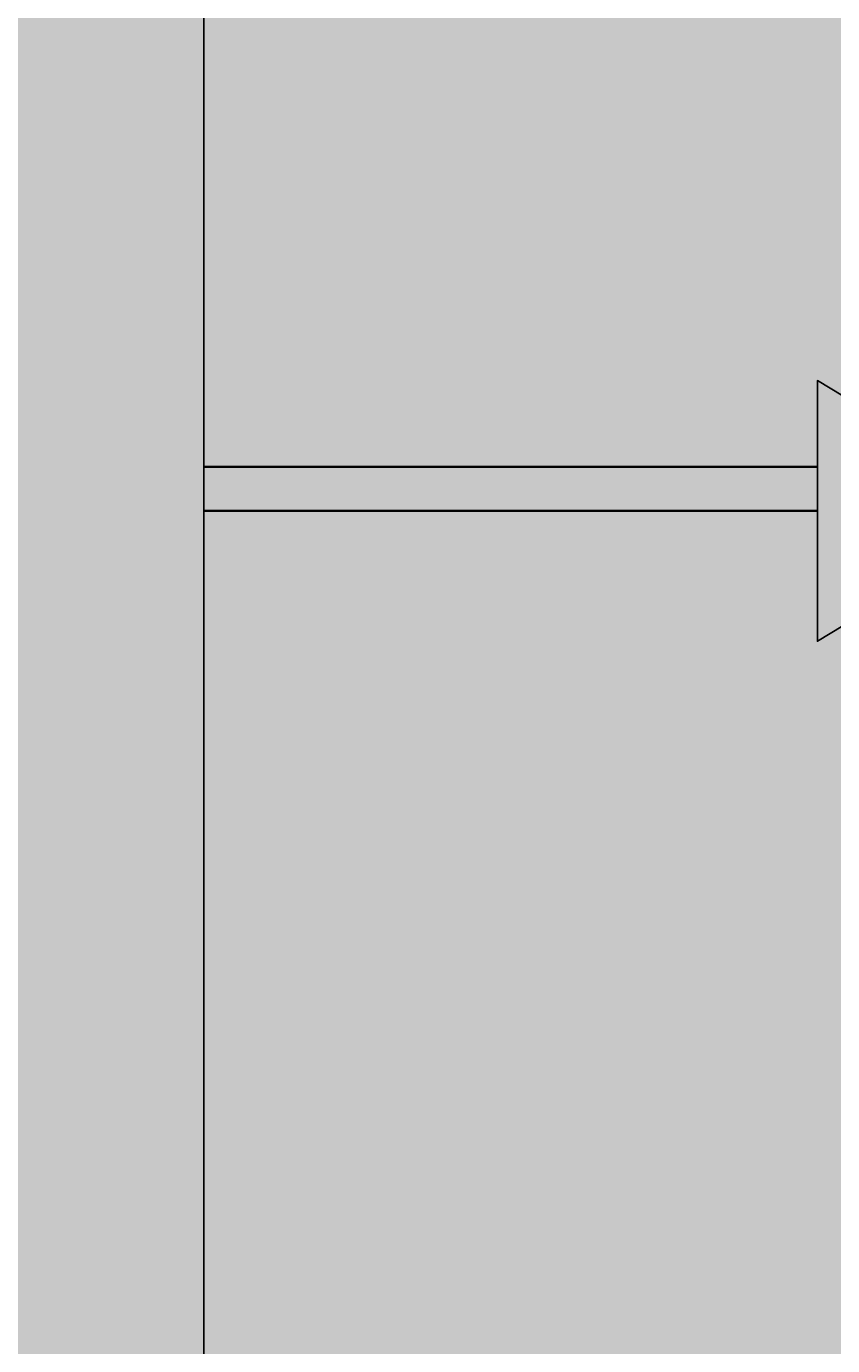
# Model space of a CAD drawing. Units: millimetres. Extents: x -22994 to 29398, y -19990 to 20176.
# Tile 57 of 135: x 198 to 216, y 65 to 95. Entities that reach past the tile are written whole.
import ezdxf
from ezdxf import colors
from ezdxf.entities.mleader import LeaderData, LeaderLine
from ezdxf.math import Vec2, Vec3

# ---------------------------------------------------------------- set-up
doc = ezdxf.new("R2010")
doc.units = ezdxf.units.MM
doc.header["$MEASUREMENT"] = 0
for name, color, linetype, lineweight in [('M-ANNO-TEXT', 7, 'Continuous', 25), ('M-DIMS', 2, 'Continuous', 18), ('M-EQPM', 7, 'Continuous', 25), ('M-EQPM-PATT', 7, 'Continuous', 18), ('M-PIPE', 7, 'Continuous', 35)]:
    doc.layers.add(name, color=color, linetype=linetype, lineweight=lineweight)
doc.styles.get("Standard").update_dxf_attribs({"font": 'arial.ttf'})
doc.dimstyles.get("Standard").update_dxf_attribs({"dimtxt": 0.18, "dimasz": 10000, "dimexe": 0.18, "dimexo": 0.0625, "dimgap": 0.09, "dimtad": 0, "dimtih": 1, "dimtoh": 1, "dimdec": 0, "dimzin": 0, "dimdsep": 46, "dimtxsty": 'Standard', "dimcen": 0.09, "dimadec": 0, "dimazin": 0, "dimtfac": 1, "dimtdec": 0, "dimtofl": 0, "dimtmove": 0, "dimatfit": 3, "dimfxl": 1, "dimtolj": 1, "dimtzin": 0, "dimlwd": 30, "dimarcsym": 0})

# ---------------------------------------------------------------- blocks, each defined once
blk = doc.blocks.new('*D2')
at = {"layer": 'Defpoints', "color": 0, "transparency": 16777216}
for p in [(6.677, 10.271), (290.852, 10.271), (290.852, -5.079)]:
    blk.add_point(p, dxfattribs=at)
at = {"layer": 'M-DIMS', "color": 0, "lineweight": -2, "transparency": 16777216}
for p, q in [((6.677, 10.209), (6.677, -5.259)), ((290.852, 10.209), (290.852, -5.259))]:
    blk.add_line(p, q, dxfattribs=at)
at = {"layer": 'M-DIMS', "color": 0, "lineweight": 30, "transparency": 16777216}
for p, q in [((-9993.323, -5.079), (-19993.323, -5.079)), ((10290.852, -5.079), (20290.852, -5.079))]:
    blk.add_line(p, q, dxfattribs=at)
at = {"layer": 'M-DIMS', "color": 0, "transparency": 16777216}
for points in [[(-9993.323, 1661.588), (-9993.323, -1671.745), (6.677, -5.079)], [(10290.852, 1661.588), (10290.852, -1671.745), (290.852, -5.079)]]:
    blk.add_solid(points, dxfattribs=at)
at = {"layer": 'M-DIMS', "color": 0, "transparency": 16777216, "insert": (148.765, -5.079), "char_height": 0.18, "attachment_point": 5}
blk.add_mtext('\\A1;284.2', dxfattribs=at)
blk = doc.blocks.new('*D3')
at = {"layer": 'Defpoints', "color": 0, "transparency": 16777216}
for p in [(110.265, 204.165), (110.265, 176.366), (95.833, 127.967)]:
    blk.add_point(p, dxfattribs=at)
at = {"layer": 'M-DIMS', "color": 0, "lineweight": -2, "transparency": 16777216}
for p, q in [((95.833, 128.03), (95.833, 204.345)), ((110.265, 176.429), (110.265, 204.345))]:
    blk.add_line(p, q, dxfattribs=at)
at = {"layer": 'M-DIMS', "color": 0, "lineweight": 30, "transparency": 16777216}
for p, q in [((-9904.167, 204.165), (-19904.167, 204.165)), ((10110.265, 204.165), (20110.265, 204.165))]:
    blk.add_line(p, q, dxfattribs=at)
at = {"layer": 'M-DIMS', "color": 0, "transparency": 16777216}
for points in [[(-9904.167, 1870.832), (-9904.167, -1462.501), (95.833, 204.165)], [(10110.265, 1870.832), (10110.265, -1462.501), (110.265, 204.165)]]:
    blk.add_solid(points, dxfattribs=at)
at = {"layer": 'M-DIMS', "color": 0, "transparency": 16777216, "insert": (103.049, 204.165), "char_height": 0.18, "attachment_point": 5}
blk.add_mtext('\\A1;14.432', dxfattribs=at)
blk = doc.blocks.new('*D4')
at = {"layer": 'Defpoints', "color": 0, "transparency": 16777216}
for p in [(116.265, 204.165), (110.265, 176.366), (116.265, 176.366)]:
    blk.add_point(p, dxfattribs=at)
at = {"layer": 'M-DIMS', "color": 0, "lineweight": -2, "transparency": 16777216}
for p, q in [((110.265, 176.429), (110.265, 204.345)), ((116.265, 176.429), (116.265, 204.345))]:
    blk.add_line(p, q, dxfattribs=at)
at = {"layer": 'M-DIMS', "color": 0, "lineweight": 30, "transparency": 16777216}
for p, q in [((-9889.735, 204.165), (-19889.735, 204.165)), ((10116.265, 204.165), (20116.265, 204.165))]:
    blk.add_line(p, q, dxfattribs=at)
at = {"layer": 'M-DIMS', "color": 0, "transparency": 16777216}
for points in [[(-9889.735, 1870.832), (-9889.735, -1462.501), (110.265, 204.165)], [(10116.265, 1870.832), (10116.265, -1462.501), (116.265, 204.165)]]:
    blk.add_solid(points, dxfattribs=at)
at = {"layer": 'M-DIMS', "color": 0, "transparency": 16777216, "insert": (113.265, 204.165), "char_height": 0.18, "attachment_point": 5}
blk.add_mtext('\\A1;6', dxfattribs=at)
blk = doc.blocks.new('*D5')
at = {"layer": 'Defpoints', "color": 0, "transparency": 16777216}
for p in [(181.265, 204.165), (116.265, 176.366), (181.265, 176.366)]:
    blk.add_point(p, dxfattribs=at)
at = {"layer": 'M-DIMS', "color": 0, "lineweight": -2, "transparency": 16777216}
for p, q in [((116.265, 176.429), (116.265, 204.345)), ((181.265, 176.429), (181.265, 204.345))]:
    blk.add_line(p, q, dxfattribs=at)
at = {"layer": 'M-DIMS', "color": 0, "lineweight": 30, "transparency": 16777216}
for p, q in [((-9883.735, 204.165), (-19883.735, 204.165)), ((10181.265, 204.165), (20181.265, 204.165))]:
    blk.add_line(p, q, dxfattribs=at)
at = {"layer": 'M-DIMS', "color": 0, "transparency": 16777216}
for points in [[(-9883.735, 1870.832), (-9883.735, -1462.501), (116.265, 204.165)], [(10181.265, 1870.832), (10181.265, -1462.501), (181.265, 204.165)]]:
    blk.add_solid(points, dxfattribs=at)
at = {"layer": 'M-DIMS', "color": 0, "transparency": 16777216, "insert": (148.765, 204.165), "char_height": 0.18, "attachment_point": 5}
blk.add_mtext('\\A1;65', dxfattribs=at)
blk = doc.blocks.new('*D6')
at = {"layer": 'Defpoints', "color": 0, "transparency": 16777216}
for p in [(187.265, 204.165), (181.265, 176.366), (187.265, 176.366)]:
    blk.add_point(p, dxfattribs=at)
at = {"layer": 'M-DIMS', "color": 0, "lineweight": -2, "transparency": 16777216}
for p, q in [((181.265, 176.429), (181.265, 204.345)), ((187.265, 176.429), (187.265, 204.345))]:
    blk.add_line(p, q, dxfattribs=at)
at = {"layer": 'M-DIMS', "color": 0, "lineweight": 30, "transparency": 16777216}
for p, q in [((-9818.735, 204.165), (-19818.735, 204.165)), ((10187.265, 204.165), (20187.265, 204.165))]:
    blk.add_line(p, q, dxfattribs=at)
at = {"layer": 'M-DIMS', "color": 0, "transparency": 16777216}
for points in [[(-9818.735, 1870.832), (-9818.735, -1462.501), (181.265, 204.165)], [(10187.265, 1870.832), (10187.265, -1462.501), (187.265, 204.165)]]:
    blk.add_solid(points, dxfattribs=at)
at = {"layer": 'M-DIMS', "color": 0, "transparency": 16777216, "insert": (184.265, 204.165), "char_height": 0.18, "attachment_point": 5}
blk.add_mtext('\\A1;6', dxfattribs=at)
blk = doc.blocks.new('*D7')
at = {"layer": 'Defpoints', "color": 0, "transparency": 16777216}
for p in [(201.697, 204.165), (187.265, 176.366), (201.697, 127.967)]:
    blk.add_point(p, dxfattribs=at)
at = {"layer": 'M-DIMS', "color": 0, "lineweight": -2, "transparency": 16777216}
for p, q in [((187.265, 176.429), (187.265, 204.345)), ((201.697, 128.03), (201.697, 204.345))]:
    blk.add_line(p, q, dxfattribs=at)
at = {"layer": 'M-DIMS', "color": 0, "lineweight": 30, "transparency": 16777216}
for p, q in [((-9812.735, 204.165), (-19812.735, 204.165)), ((10201.697, 204.165), (20201.697, 204.165))]:
    blk.add_line(p, q, dxfattribs=at)
at = {"layer": 'M-DIMS', "color": 0, "transparency": 16777216}
for points in [[(-9812.735, 1870.832), (-9812.735, -1462.501), (187.265, 204.165)], [(10201.697, 1870.832), (10201.697, -1462.501), (201.697, 204.165)]]:
    blk.add_solid(points, dxfattribs=at)
at = {"layer": 'M-DIMS', "color": 0, "transparency": 16777216, "insert": (194.481, 204.165), "char_height": 0.18, "attachment_point": 5}
blk.add_mtext('\\A1;14.432', dxfattribs=at)
blk = doc.blocks.new('*D8')
at = {"layer": 'Defpoints', "color": 0, "transparency": 16777216}
for p in [(227.648, 204.165), (227.648, 146.73), (201.697, 127.967)]:
    blk.add_point(p, dxfattribs=at)
at = {"layer": 'M-DIMS', "color": 0, "lineweight": -2, "transparency": 16777216}
for p, q in [((201.697, 128.03), (201.697, 204.345)), ((227.648, 146.792), (227.648, 204.345))]:
    blk.add_line(p, q, dxfattribs=at)
at = {"layer": 'M-DIMS', "color": 0, "lineweight": 30, "transparency": 16777216}
for p, q in [((-9798.303, 204.165), (-19798.303, 204.165)), ((10227.648, 204.165), (20227.648, 204.165))]:
    blk.add_line(p, q, dxfattribs=at)
at = {"layer": 'M-DIMS', "color": 0, "transparency": 16777216}
for points in [[(-9798.303, 1870.832), (-9798.303, -1462.501), (201.697, 204.165)], [(10227.648, 1870.832), (10227.648, -1462.501), (227.648, 204.165)]]:
    blk.add_solid(points, dxfattribs=at)
at = {"layer": 'M-DIMS', "color": 0, "transparency": 16777216, "insert": (214.673, 204.165), "char_height": 0.18, "attachment_point": 5}
blk.add_mtext('\\A1;25.95', dxfattribs=at)
blk = doc.blocks.new('*D9')
at = {"layer": 'Defpoints', "color": 0, "transparency": 16777216}
for p in [(187.265, 176.366), (306.202, 176.366), (290.852, 10.271)]:
    blk.add_point(p, dxfattribs=at)
at = {"layer": 'M-DIMS', "color": 0, "lineweight": 30, "transparency": 16777216}
for p, q in [((306.202, 10176.366), (306.202, 20176.366)), ((306.202, -9989.729), (306.202, -19989.729))]:
    blk.add_line(p, q, dxfattribs=at)
at = {"layer": 'M-DIMS', "color": 0, "lineweight": -2, "transparency": 16777216}
for p, q in [((187.327, 176.366), (306.382, 176.366)), ((290.915, 10.271), (306.382, 10.271))]:
    blk.add_line(p, q, dxfattribs=at)
at = {"layer": 'M-DIMS', "color": 0, "transparency": 16777216}
for points in [[(-1360.465, 10176.366), (1972.869, 10176.366), (306.202, 176.366)], [(-1360.465, -9989.729), (1972.869, -9989.729), (306.202, 10.271)]]:
    blk.add_solid(points, dxfattribs=at)
at = {"layer": 'M-DIMS', "color": 0, "transparency": 16777216, "insert": (306.202, 93.319), "char_height": 0.18, "attachment_point": 5}
blk.add_mtext('\\A1;166.1', dxfattribs=at)
blk = doc.blocks.new('*D10')
at = {"layer": 'Defpoints', "color": 0, "transparency": 16777216}
for p in [(125.65, 136.071), (133.346, 136.071), (133.346, -5.079)]:
    blk.add_point(p, dxfattribs=at)
at = {"layer": 'M-DIMS', "color": 0, "lineweight": -2, "transparency": 16777216}
for p, q in [((125.65, 136.009), (125.65, -5.259)), ((133.346, 136.009), (133.346, -5.259))]:
    blk.add_line(p, q, dxfattribs=at)
at = {"layer": 'M-DIMS', "color": 0, "lineweight": 30, "transparency": 16777216}
for p, q in [((-9874.35, -5.079), (-19874.35, -5.079)), ((10133.346, -5.079), (20133.346, -5.079))]:
    blk.add_line(p, q, dxfattribs=at)
at = {"layer": 'M-DIMS', "color": 0, "transparency": 16777216}
for points in [[(-9874.35, 1661.588), (-9874.35, -1671.745), (125.65, -5.079)], [(10133.346, 1661.588), (10133.346, -1671.745), (133.346, -5.079)]]:
    blk.add_solid(points, dxfattribs=at)
at = {"layer": 'M-DIMS', "color": 0, "transparency": 16777216, "insert": (129.498, -5.079), "char_height": 0.18, "attachment_point": 5}
blk.add_mtext('\\A1;7.696', dxfattribs=at)
blk = doc.blocks.new('*D11')
at = {"layer": 'Defpoints', "color": 0, "transparency": 16777216}
for p in [(133.346, 136.071), (135.65, 136.071), (135.65, -5.079)]:
    blk.add_point(p, dxfattribs=at)
at = {"layer": 'M-DIMS', "color": 0, "lineweight": -2, "transparency": 16777216}
for p, q in [((133.346, 136.009), (133.346, -5.259)), ((135.65, 136.009), (135.65, -5.259))]:
    blk.add_line(p, q, dxfattribs=at)
at = {"layer": 'M-DIMS', "color": 0, "lineweight": 30, "transparency": 16777216}
for p, q in [((-9866.654, -5.079), (-19866.654, -5.079)), ((10135.65, -5.079), (20135.65, -5.079))]:
    blk.add_line(p, q, dxfattribs=at)
at = {"layer": 'M-DIMS', "color": 0, "transparency": 16777216}
for points in [[(-9866.654, 1661.588), (-9866.654, -1671.745), (133.346, -5.079)], [(10135.65, 1661.588), (10135.65, -1671.745), (135.65, -5.079)]]:
    blk.add_solid(points, dxfattribs=at)
at = {"layer": 'M-DIMS', "color": 0, "transparency": 16777216, "insert": (134.498, -5.079), "char_height": 0.18, "attachment_point": 5}
blk.add_mtext('\\A1;2.304', dxfattribs=at)
blk = doc.blocks.new('*D12')
at = {"layer": 'Defpoints', "color": 0, "transparency": 16777216}
for p in [(135.65, 136.071), (145.65, 136.071), (145.65, -5.079)]:
    blk.add_point(p, dxfattribs=at)
at = {"layer": 'M-DIMS', "color": 0, "lineweight": -2, "transparency": 16777216}
for p, q in [((135.65, 136.009), (135.65, -5.259)), ((145.65, 136.009), (145.65, -5.259))]:
    blk.add_line(p, q, dxfattribs=at)
at = {"layer": 'M-DIMS', "color": 0, "lineweight": 30, "transparency": 16777216}
for p, q in [((-9864.35, -5.079), (-19864.35, -5.079)), ((10145.65, -5.079), (20145.65, -5.079))]:
    blk.add_line(p, q, dxfattribs=at)
at = {"layer": 'M-DIMS', "color": 0, "transparency": 16777216}
for points in [[(-9864.35, 1661.588), (-9864.35, -1671.745), (135.65, -5.079)], [(10145.65, 1661.588), (10145.65, -1671.745), (145.65, -5.079)]]:
    blk.add_solid(points, dxfattribs=at)
at = {"layer": 'M-DIMS', "color": 0, "transparency": 16777216, "insert": (140.65, -5.079), "char_height": 0.18, "attachment_point": 5}
blk.add_mtext('\\A1;10', dxfattribs=at)
blk = doc.blocks.new('*D13')
at = {"layer": 'Defpoints', "color": 0, "transparency": 16777216}
for p in [(145.65, 136.071), (155.65, 136.071), (155.65, -5.079)]:
    blk.add_point(p, dxfattribs=at)
at = {"layer": 'M-DIMS', "color": 0, "lineweight": -2, "transparency": 16777216}
for p, q in [((145.65, 136.009), (145.65, -5.259)), ((155.65, 136.009), (155.65, -5.259))]:
    blk.add_line(p, q, dxfattribs=at)
at = {"layer": 'M-DIMS', "color": 0, "lineweight": 30, "transparency": 16777216}
for p, q in [((-9854.35, -5.079), (-19854.35, -5.079)), ((10155.65, -5.079), (20155.65, -5.079))]:
    blk.add_line(p, q, dxfattribs=at)
at = {"layer": 'M-DIMS', "color": 0, "transparency": 16777216}
for points in [[(-9854.35, 1661.588), (-9854.35, -1671.745), (145.65, -5.079)], [(10155.65, 1661.588), (10155.65, -1671.745), (155.65, -5.079)]]:
    blk.add_solid(points, dxfattribs=at)
at = {"layer": 'M-DIMS', "color": 0, "transparency": 16777216, "insert": (150.65, -5.079), "char_height": 0.18, "attachment_point": 5}
blk.add_mtext('\\A1;10', dxfattribs=at)
blk = doc.blocks.new('*D14')
at = {"layer": 'Defpoints', "color": 0, "transparency": 16777216}
for p in [(155.65, 136.071), (165.65, 136.071), (165.65, -5.079)]:
    blk.add_point(p, dxfattribs=at)
at = {"layer": 'M-DIMS', "color": 0, "lineweight": -2, "transparency": 16777216}
for p, q in [((155.65, 136.009), (155.65, -5.259)), ((165.65, 136.009), (165.65, -5.259))]:
    blk.add_line(p, q, dxfattribs=at)
at = {"layer": 'M-DIMS', "color": 0, "lineweight": 30, "transparency": 16777216}
for p, q in [((-9844.35, -5.079), (-19844.35, -5.079)), ((10165.65, -5.079), (20165.65, -5.079))]:
    blk.add_line(p, q, dxfattribs=at)
at = {"layer": 'M-DIMS', "color": 0, "transparency": 16777216}
for points in [[(-9844.35, 1661.588), (-9844.35, -1671.745), (155.65, -5.079)], [(10165.65, 1661.588), (10165.65, -1671.745), (165.65, -5.079)]]:
    blk.add_solid(points, dxfattribs=at)
at = {"layer": 'M-DIMS', "color": 0, "transparency": 16777216, "insert": (160.65, -5.079), "char_height": 0.18, "attachment_point": 5}
blk.add_mtext('\\A1;10', dxfattribs=at)
blk = doc.blocks.new('*D15')
at = {"layer": 'Defpoints', "color": 0, "transparency": 16777216}
for p in [(173.346, 154.788), (173.346, 136.071), (306.202, 136.071)]:
    blk.add_point(p, dxfattribs=at)
at = {"layer": 'M-DIMS', "color": 0, "lineweight": 30, "transparency": 16777216}
for p, q in [((306.202, 10154.788), (306.202, 20154.788)), ((306.202, -9863.929), (306.202, -19863.929))]:
    blk.add_line(p, q, dxfattribs=at)
at = {"layer": 'M-DIMS', "color": 0, "lineweight": -2, "transparency": 16777216}
for p, q in [((173.408, 154.788), (306.382, 154.788)), ((173.408, 136.071), (306.382, 136.071))]:
    blk.add_line(p, q, dxfattribs=at)
at = {"layer": 'M-DIMS', "color": 0, "transparency": 16777216}
for points in [[(-1360.465, 10154.788), (1972.869, 10154.788), (306.202, 154.788)], [(-1360.465, -9863.929), (1972.869, -9863.929), (306.202, 136.071)]]:
    blk.add_solid(points, dxfattribs=at)
at = {"layer": 'M-DIMS', "color": 0, "transparency": 16777216, "insert": (306.202, 145.43), "char_height": 0.18, "attachment_point": 5}
blk.add_mtext('\\A1;18.717', dxfattribs=at)
blk = doc.blocks.new('*D16')
at = {"layer": 'Defpoints', "color": 0, "transparency": 16777216}
for p in [(120.17, 204.165), (110.466, 48.035), (120.17, 48.035)]:
    blk.add_point(p, dxfattribs=at)
at = {"layer": 'M-DIMS', "color": 0, "lineweight": -2, "transparency": 16777216}
for p, q in [((110.466, 48.097), (110.466, 204.345)), ((120.17, 48.097), (120.17, 204.345))]:
    blk.add_line(p, q, dxfattribs=at)
at = {"layer": 'M-DIMS', "color": 0, "lineweight": 30, "transparency": 16777216}
for p, q in [((-9889.534, 204.165), (-19889.534, 204.165)), ((10120.17, 204.165), (20120.17, 204.165))]:
    blk.add_line(p, q, dxfattribs=at)
at = {"layer": 'M-DIMS', "color": 0, "transparency": 16777216}
for points in [[(-9889.534, 1870.832), (-9889.534, -1462.501), (110.466, 204.165)], [(10120.17, 1870.832), (10120.17, -1462.501), (120.17, 204.165)]]:
    blk.add_solid(points, dxfattribs=at)
at = {"layer": 'M-DIMS', "color": 0, "transparency": 16777216, "insert": (115.318, 204.165), "char_height": 0.18, "attachment_point": 5}
blk.add_mtext('\\A1;9.704', dxfattribs=at)
blk = doc.blocks.new('*D17')
at = {"layer": 'Defpoints', "color": 0, "transparency": 16777216}
for p in [(126.17, 204.165), (120.17, 48.035), (126.17, 48.035)]:
    blk.add_point(p, dxfattribs=at)
at = {"layer": 'M-DIMS', "color": 0, "lineweight": -2, "transparency": 16777216}
for p, q in [((120.17, 48.097), (120.17, 204.345)), ((126.17, 48.097), (126.17, 204.345))]:
    blk.add_line(p, q, dxfattribs=at)
at = {"layer": 'M-DIMS', "color": 0, "lineweight": 30, "transparency": 16777216}
for p, q in [((-9879.83, 204.165), (-19879.83, 204.165)), ((10126.17, 204.165), (20126.17, 204.165))]:
    blk.add_line(p, q, dxfattribs=at)
at = {"layer": 'M-DIMS', "color": 0, "transparency": 16777216}
for points in [[(-9879.83, 1870.832), (-9879.83, -1462.501), (120.17, 204.165)], [(10126.17, 1870.832), (10126.17, -1462.501), (126.17, 204.165)]]:
    blk.add_solid(points, dxfattribs=at)
at = {"layer": 'M-DIMS', "color": 0, "transparency": 16777216, "insert": (123.17, 204.165), "char_height": 0.18, "attachment_point": 5}
blk.add_mtext('\\A1;6', dxfattribs=at)
blk = doc.blocks.new('*D18')
at = {"layer": 'Defpoints', "color": 0, "transparency": 16777216}
for p in [(132.17, 204.165), (126.17, 48.035), (132.17, 48.035)]:
    blk.add_point(p, dxfattribs=at)
at = {"layer": 'M-DIMS', "color": 0, "lineweight": -2, "transparency": 16777216}
for p, q in [((126.17, 48.097), (126.17, 204.345)), ((132.17, 48.097), (132.17, 204.345))]:
    blk.add_line(p, q, dxfattribs=at)
at = {"layer": 'M-DIMS', "color": 0, "lineweight": 30, "transparency": 16777216}
for p, q in [((-9873.83, 204.165), (-19873.83, 204.165)), ((10132.17, 204.165), (20132.17, 204.165))]:
    blk.add_line(p, q, dxfattribs=at)
at = {"layer": 'M-DIMS', "color": 0, "transparency": 16777216}
for points in [[(-9873.83, 1870.832), (-9873.83, -1462.501), (126.17, 204.165)], [(10132.17, 1870.832), (10132.17, -1462.501), (132.17, 204.165)]]:
    blk.add_solid(points, dxfattribs=at)
at = {"layer": 'M-DIMS', "color": 0, "transparency": 16777216, "insert": (129.17, 204.165), "char_height": 0.18, "attachment_point": 5}
blk.add_mtext('\\A1;6', dxfattribs=at)
blk = doc.blocks.new('*D19')
at = {"layer": 'Defpoints', "color": 0, "transparency": 16777216}
for p in [(138.17, 204.165), (132.17, 48.035), (138.17, 48.035)]:
    blk.add_point(p, dxfattribs=at)
at = {"layer": 'M-DIMS', "color": 0, "lineweight": -2, "transparency": 16777216}
for p, q in [((132.17, 48.097), (132.17, 204.345)), ((138.17, 48.097), (138.17, 204.345))]:
    blk.add_line(p, q, dxfattribs=at)
at = {"layer": 'M-DIMS', "color": 0, "lineweight": 30, "transparency": 16777216}
for p, q in [((-9867.83, 204.165), (-19867.83, 204.165)), ((10138.17, 204.165), (20138.17, 204.165))]:
    blk.add_line(p, q, dxfattribs=at)
at = {"layer": 'M-DIMS', "color": 0, "transparency": 16777216}
for points in [[(-9867.83, 1870.832), (-9867.83, -1462.501), (132.17, 204.165)], [(10138.17, 1870.832), (10138.17, -1462.501), (138.17, 204.165)]]:
    blk.add_solid(points, dxfattribs=at)
at = {"layer": 'M-DIMS', "color": 0, "transparency": 16777216, "insert": (135.17, 204.165), "char_height": 0.18, "attachment_point": 5}
blk.add_mtext('\\A1;6', dxfattribs=at)
blk = doc.blocks.new('*D20')
at = {"layer": 'Defpoints', "color": 0, "transparency": 16777216}
for p in [(144.17, 204.165), (138.17, 48.035), (144.17, 48.035)]:
    blk.add_point(p, dxfattribs=at)
at = {"layer": 'M-DIMS', "color": 0, "lineweight": -2, "transparency": 16777216}
for p, q in [((138.17, 48.097), (138.17, 204.345)), ((144.17, 48.097), (144.17, 204.345))]:
    blk.add_line(p, q, dxfattribs=at)
at = {"layer": 'M-DIMS', "color": 0, "lineweight": 30, "transparency": 16777216}
for p, q in [((-9861.83, 204.165), (-19861.83, 204.165)), ((10144.17, 204.165), (20144.17, 204.165))]:
    blk.add_line(p, q, dxfattribs=at)
at = {"layer": 'M-DIMS', "color": 0, "transparency": 16777216}
for points in [[(-9861.83, 1870.832), (-9861.83, -1462.501), (138.17, 204.165)], [(10144.17, 1870.832), (10144.17, -1462.501), (144.17, 204.165)]]:
    blk.add_solid(points, dxfattribs=at)
at = {"layer": 'M-DIMS', "color": 0, "transparency": 16777216, "insert": (141.17, 204.165), "char_height": 0.18, "attachment_point": 5}
blk.add_mtext('\\A1;6', dxfattribs=at)
blk = doc.blocks.new('*D21')
at = {"layer": 'Defpoints', "color": 0, "transparency": 16777216}
for p in [(149.116, 204.165), (144.17, 48.035), (149.116, 48.035)]:
    blk.add_point(p, dxfattribs=at)
at = {"layer": 'M-DIMS', "color": 0, "lineweight": -2, "transparency": 16777216}
for p, q in [((144.17, 48.097), (144.17, 204.345)), ((149.116, 48.097), (149.116, 204.345))]:
    blk.add_line(p, q, dxfattribs=at)
at = {"layer": 'M-DIMS', "color": 0, "lineweight": 30, "transparency": 16777216}
for p, q in [((-9855.83, 204.165), (-19855.83, 204.165)), ((10149.116, 204.165), (20149.116, 204.165))]:
    blk.add_line(p, q, dxfattribs=at)
at = {"layer": 'M-DIMS', "color": 0, "transparency": 16777216}
for points in [[(-9855.83, 1870.832), (-9855.83, -1462.501), (144.17, 204.165)], [(10149.116, 1870.832), (10149.116, -1462.501), (149.116, 204.165)]]:
    blk.add_solid(points, dxfattribs=at)
at = {"layer": 'M-DIMS', "color": 0, "transparency": 16777216, "insert": (146.643, 204.165), "char_height": 0.18, "attachment_point": 5}
blk.add_mtext('\\A1;4.945', dxfattribs=at)
blk = doc.blocks.new('*D22')
at = {"layer": 'Defpoints', "color": 0, "transparency": 16777216}
for p in [(149.116, 30.99), (155.116, 30.99), (155.116, -5.079)]:
    blk.add_point(p, dxfattribs=at)
at = {"layer": 'M-DIMS', "color": 0, "lineweight": -2, "transparency": 16777216}
for p, q in [((149.116, 30.927), (149.116, -5.259)), ((155.116, 30.927), (155.116, -5.259))]:
    blk.add_line(p, q, dxfattribs=at)
at = {"layer": 'M-DIMS', "color": 0, "lineweight": 30, "transparency": 16777216}
for p, q in [((-9850.884, -5.079), (-19850.884, -5.079)), ((10155.116, -5.079), (20155.116, -5.079))]:
    blk.add_line(p, q, dxfattribs=at)
at = {"layer": 'M-DIMS', "color": 0, "transparency": 16777216}
for points in [[(-9850.884, 1661.588), (-9850.884, -1671.745), (149.116, -5.079)], [(10155.116, 1661.588), (10155.116, -1671.745), (155.116, -5.079)]]:
    blk.add_solid(points, dxfattribs=at)
at = {"layer": 'M-DIMS', "color": 0, "transparency": 16777216, "insert": (152.116, -5.079), "char_height": 0.18, "attachment_point": 5}
blk.add_mtext('\\A1;6', dxfattribs=at)
blk = doc.blocks.new('*D23')
at = {"layer": 'Defpoints', "color": 0, "transparency": 16777216}
for p in [(155.116, 30.99), (161.116, 30.99), (161.116, -5.079)]:
    blk.add_point(p, dxfattribs=at)
at = {"layer": 'M-DIMS', "color": 0, "lineweight": -2, "transparency": 16777216}
for p, q in [((155.116, 30.927), (155.116, -5.259)), ((161.116, 30.927), (161.116, -5.259))]:
    blk.add_line(p, q, dxfattribs=at)
at = {"layer": 'M-DIMS', "color": 0, "lineweight": 30, "transparency": 16777216}
for p, q in [((-9844.884, -5.079), (-19844.884, -5.079)), ((10161.116, -5.079), (20161.116, -5.079))]:
    blk.add_line(p, q, dxfattribs=at)
at = {"layer": 'M-DIMS', "color": 0, "transparency": 16777216}
for points in [[(-9844.884, 1661.588), (-9844.884, -1671.745), (155.116, -5.079)], [(10161.116, 1661.588), (10161.116, -1671.745), (161.116, -5.079)]]:
    blk.add_solid(points, dxfattribs=at)
at = {"layer": 'M-DIMS', "color": 0, "transparency": 16777216, "insert": (158.116, -5.079), "char_height": 0.18, "attachment_point": 5}
blk.add_mtext('\\A1;6', dxfattribs=at)
blk = doc.blocks.new('*D24')
at = {"layer": 'Defpoints', "color": 0, "transparency": 16777216}
for p in [(161.116, 30.99), (166.439, 30.99), (166.439, -5.079)]:
    blk.add_point(p, dxfattribs=at)
at = {"layer": 'M-DIMS', "color": 0, "lineweight": -2, "transparency": 16777216}
for p, q in [((161.116, 30.927), (161.116, -5.259)), ((166.439, 30.927), (166.439, -5.259))]:
    blk.add_line(p, q, dxfattribs=at)
at = {"layer": 'M-DIMS', "color": 0, "lineweight": 30, "transparency": 16777216}
for p, q in [((-9838.884, -5.079), (-19838.884, -5.079)), ((10166.439, -5.079), (20166.439, -5.079))]:
    blk.add_line(p, q, dxfattribs=at)
at = {"layer": 'M-DIMS', "color": 0, "transparency": 16777216}
for points in [[(-9838.884, 1661.588), (-9838.884, -1671.745), (161.116, -5.079)], [(10166.439, 1661.588), (10166.439, -1671.745), (166.439, -5.079)]]:
    blk.add_solid(points, dxfattribs=at)
at = {"layer": 'M-DIMS', "color": 0, "transparency": 16777216, "insert": (163.777, -5.079), "char_height": 0.18, "attachment_point": 5}
blk.add_mtext('\\A1;5.323', dxfattribs=at)
blk = doc.blocks.new('*D25')
at = {"layer": 'Defpoints', "color": 0, "transparency": 16777216}
for p in [(166.439, 30.99), (172.439, 30.99), (172.439, -5.079)]:
    blk.add_point(p, dxfattribs=at)
at = {"layer": 'M-DIMS', "color": 0, "lineweight": -2, "transparency": 16777216}
for p, q in [((166.439, 30.927), (166.439, -5.259)), ((172.439, 30.927), (172.439, -5.259))]:
    blk.add_line(p, q, dxfattribs=at)
at = {"layer": 'M-DIMS', "color": 0, "lineweight": 30, "transparency": 16777216}
for p, q in [((-9833.561, -5.079), (-19833.561, -5.079)), ((10172.439, -5.079), (20172.439, -5.079))]:
    blk.add_line(p, q, dxfattribs=at)
at = {"layer": 'M-DIMS', "color": 0, "transparency": 16777216}
for points in [[(-9833.561, 1661.588), (-9833.561, -1671.745), (166.439, -5.079)], [(10172.439, 1661.588), (10172.439, -1671.745), (172.439, -5.079)]]:
    blk.add_solid(points, dxfattribs=at)
at = {"layer": 'M-DIMS', "color": 0, "transparency": 16777216, "insert": (169.439, -5.079), "char_height": 0.18, "attachment_point": 5}
blk.add_mtext('\\A1;6', dxfattribs=at)
blk = doc.blocks.new('*D26')
at = {"layer": 'Defpoints', "color": 0, "transparency": 16777216}
for p in [(172.439, 30.99), (178.439, 30.99), (178.439, -5.079)]:
    blk.add_point(p, dxfattribs=at)
at = {"layer": 'M-DIMS', "color": 0, "lineweight": -2, "transparency": 16777216}
for p, q in [((172.439, 30.927), (172.439, -5.259)), ((178.439, 30.927), (178.439, -5.259))]:
    blk.add_line(p, q, dxfattribs=at)
at = {"layer": 'M-DIMS', "color": 0, "lineweight": 30, "transparency": 16777216}
for p, q in [((-9827.561, -5.079), (-19827.561, -5.079)), ((10178.439, -5.079), (20178.439, -5.079))]:
    blk.add_line(p, q, dxfattribs=at)
at = {"layer": 'M-DIMS', "color": 0, "transparency": 16777216}
for points in [[(-9827.561, 1661.588), (-9827.561, -1671.745), (172.439, -5.079)], [(10178.439, 1661.588), (10178.439, -1671.745), (178.439, -5.079)]]:
    blk.add_solid(points, dxfattribs=at)
at = {"layer": 'M-DIMS', "color": 0, "transparency": 16777216, "insert": (175.439, -5.079), "char_height": 0.18, "attachment_point": 5}
blk.add_mtext('\\A1;6', dxfattribs=at)
blk = doc.blocks.new('*D27')
at = {"layer": 'Defpoints', "color": 0, "transparency": 16777216}
for p in [(178.439, 30.99), (188.117, 30.99), (188.117, -5.079)]:
    blk.add_point(p, dxfattribs=at)
at = {"layer": 'M-DIMS', "color": 0, "lineweight": -2, "transparency": 16777216}
for p, q in [((178.439, 30.927), (178.439, -5.259)), ((188.117, 30.927), (188.117, -5.259))]:
    blk.add_line(p, q, dxfattribs=at)
at = {"layer": 'M-DIMS', "color": 0, "lineweight": 30, "transparency": 16777216}
for p, q in [((-9821.561, -5.079), (-19821.561, -5.079)), ((10188.117, -5.079), (20188.117, -5.079))]:
    blk.add_line(p, q, dxfattribs=at)
at = {"layer": 'M-DIMS', "color": 0, "transparency": 16777216}
for points in [[(-9821.561, 1661.588), (-9821.561, -1671.745), (178.439, -5.079)], [(10188.117, 1661.588), (10188.117, -1671.745), (188.117, -5.079)]]:
    blk.add_solid(points, dxfattribs=at)
at = {"layer": 'M-DIMS', "color": 0, "transparency": 16777216, "insert": (183.278, -5.079), "char_height": 0.18, "attachment_point": 5}
blk.add_mtext('\\A1;9.679', dxfattribs=at)
blk = doc.blocks.new('*D28')
at = {"layer": 'Defpoints', "color": 0, "transparency": 16777216}
for p in [(188.117, 48.035), (306.202, 48.035), (188.117, 30.99)]:
    blk.add_point(p, dxfattribs=at)
at = {"layer": 'M-DIMS', "color": 0, "lineweight": 30, "transparency": 16777216}
for p, q in [((306.202, 10048.035), (306.202, 20048.035)), ((306.202, -9969.01), (306.202, -19969.01))]:
    blk.add_line(p, q, dxfattribs=at)
at = {"layer": 'M-DIMS', "color": 0, "lineweight": -2, "transparency": 16777216}
for p, q in [((188.18, 48.035), (306.382, 48.035)), ((188.18, 30.99), (306.382, 30.99))]:
    blk.add_line(p, q, dxfattribs=at)
at = {"layer": 'M-DIMS', "color": 0, "transparency": 16777216}
for points in [[(-1360.465, 10048.035), (1972.869, 10048.035), (306.202, 48.035)], [(-1360.465, -9969.01), (1972.869, -9969.01), (306.202, 30.99)]]:
    blk.add_solid(points, dxfattribs=at)
at = {"layer": 'M-DIMS', "color": 0, "transparency": 16777216, "insert": (306.202, 39.512), "char_height": 0.18, "attachment_point": 5}
blk.add_mtext('\\A1;17.045', dxfattribs=at)
blk = doc.blocks.new('*D29')
at = {"layer": 'Defpoints', "color": 0, "transparency": 16777216}
for p in [(36.801, 80.045), (64.03, 80.045)]:
    blk.add_point(p, dxfattribs=at)
at = {"layer": 'M-DIMS', "color": 0, "lineweight": -2, "transparency": 16777216}
for p, q in [((50.325, 80.045), (50.505, 80.045)), ((50.415, 79.955), (50.415, 80.135))]:
    blk.add_line(p, q, dxfattribs=at)
at = {"layer": 'M-DIMS', "color": 0, "lineweight": 30, "transparency": 16777216}
blk.add_line((20064.03, 80.03), (10064.03, 80.038), dxfattribs=at)
at = {"layer": 'M-DIMS', "color": 0, "transparency": 16777216}
blk.add_solid([(10064.031, 1746.704), (10064.028, -1586.629), (64.03, 80.045)], dxfattribs=at)
at = {"layer": 'M-DIMS', "color": 0, "transparency": 16777216, "insert": (20064.521, 80.03), "char_height": 0.18, "attachment_point": 5}
blk.add_mtext('\\A1;∅27.23', dxfattribs=at)
blk = doc.blocks.new('*D36')
at = {"layer": 'Defpoints', "color": 0, "transparency": 16777216}
for p in [(46.39, 31.303), (46.387, 26.593)]:
    blk.add_point(p, dxfattribs=at)
at = {"layer": 'M-DIMS', "color": 0, "lineweight": 30, "transparency": 16777216}
for p, q in [((57.15, 20031.301), (51.77, 10031.302)), ((10057.15, 20031.301), (57.15, 20031.301))]:
    blk.add_line(p, q, dxfattribs=at)
at = {"layer": 'M-DIMS', "color": 0, "lineweight": -2, "transparency": 16777216}
for p, q in [((46.299, 28.948), (46.479, 28.948)), ((46.389, 28.858), (46.389, 29.038))]:
    blk.add_line(p, q, dxfattribs=at)
at = {"layer": 'M-DIMS', "color": 0, "transparency": 16777216}
blk.add_solid([(-1614.896, 10032.199), (1718.436, 10030.405), (46.39, 31.303)], dxfattribs=at)
at = {"layer": 'M-DIMS', "color": 0, "transparency": 16777216, "insert": (10057.554, 20031.301), "char_height": 0.18, "attachment_point": 5}
blk.add_mtext('\\A1;∅4.71', dxfattribs=at)
blk = doc.blocks.new('*D37')
at = {"layer": 'Defpoints', "color": 0, "transparency": 16777216}
for p in [(54.834, 118.615), (59.494, 118.614)]:
    blk.add_point(p, dxfattribs=at)
at = {"layer": 'M-DIMS', "color": 0, "lineweight": -2, "transparency": 16777216}
for p, q in [((57.074, 118.614), (57.254, 118.614)), ((57.164, 118.524), (57.164, 118.704))]:
    blk.add_line(p, q, dxfattribs=at)
at = {"layer": 'M-DIMS', "color": 0, "lineweight": 30, "transparency": 16777216}
blk.add_line((20059.493, 116.253), (10059.494, 117.434), dxfattribs=at)
at = {"layer": 'M-DIMS', "color": 0, "transparency": 16777216}
blk.add_solid([(10059.69, 1784.1), (10059.297, -1549.233), (59.494, 118.614)], dxfattribs=at)
at = {"layer": 'M-DIMS', "color": 0, "transparency": 16777216, "insert": (20059.985, 116.253), "char_height": 0.18, "attachment_point": 5}
blk.add_mtext('\\A1;∅4.659', dxfattribs=at)

msp = doc.modelspace()

# ---------------------------------------------------------------- hatches: boundary and pattern name
at = {"layer": 'M-EQPM-PATT'}
h = msp.add_hatch(color=256, dxfattribs=at)
h.set_gradient(color1=(205, 32, 39), color2=(205, 32, 39), tint=1)
h.paths.add_polyline_path([(116.2647, 150.3662), (116.2647, 170.3662), (116.2647, 176.3662), (110.2647, 176.3662), (110.2647, 152.0276), (95.8327, 127.967), (95.8327, 16.6063), (201.6967, 16.6063), (201.6967, 127.967), (187.2647, 152.0276), (187.2647, 176.3662), (181.2647, 176.3662), (181.2647, 170.3662), (181.2647, 150.3662), (195.6967, 126.3055), (195.6967, 22.6063), (101.8327, 22.6063), (101.8327, 126.3055)])
h.paths.add_polyline_path([(185.2208, 88.6347), (101.8327, 88.6347), (101.8327, 87.6347), (182.8066, 87.6347), (178.7313, 83.5594), (195.6967, 83.5594), (195.6967, 84.5594), (181.1455, 84.5594)], flags=17)
h.paths.add_polyline_path([(95.8327, 88.6347), (60.9779, 88.6347, -0.0228552), (61.7178, 87.6347), (95.8327, 87.6347)])
h.paths.add_polyline_path([(215.6212, 86.5189), (215.6212, 80.5999), (220.5095, 83.5594)])
h.paths.add_polyline_path([(215.6212, 84.5594), (201.6967, 84.5594), (201.6967, 83.5594), (215.6212, 83.5594)])
h.paths.add_polyline_path([(225.3978, 86.5189), (220.5095, 83.5594), (225.3978, 80.5999)])
h.paths.add_polyline_path([(231.6256, 84.5594), (225.3978, 84.5594), (225.3978, 83.5594), (231.6256, 83.5594)])

# ---------------------------------------------------------------- linework, layer by layer
at = {"layer": 'M-EQPM'}
for points in [[(110.2647, 176.3662), (110.2647, 152.0276), (95.8327, 127.967), (95.8327, 16.6063), (201.6967, 16.6063), (201.6967, 127.967), (187.2647, 152.0276), (187.2647, 176.3662)], [(225.3978, 86.5189), (215.6212, 80.5999), (215.6212, 86.5189), (225.3978, 80.5999)]]:
    msp.add_lwpolyline(points, close=True, dxfattribs=at)
at = {"layer": 'M-PIPE'}
for p, q in [((201.6967, 84.5594), (215.6212, 84.5594)), ((201.6967, 83.5594), (215.6212, 83.5594))]:
    msp.add_line(p, q, dxfattribs=at)

# ---------------------------------------------------------------- dimensions: what is measured, and where the dimension line sits
at = {"layer": 'M-DIMS'}
for base, p1, p2, override, picture, middle in [((306.202, 176.3662), (290.852, 10.2713), (187.2647, 176.3662), {"dimdec": 1, "dimlfac": 1, "dimrnd": 0, "dimzin": 0, "dimdsep": 46, "dimlunit": 2}, '*D9', (306.202, 93.3187)), ((306.202, 136.0713), (173.3459, 154.788), (173.3459, 136.0713), {"dimdec": 3, "dimlfac": 1, "dimrnd": 0, "dimzin": 0, "dimdsep": 46, "dimlunit": 2}, '*D15', (306.202, 145.4297)), ((306.202, 48.0349), (188.1175, 30.9895), (188.1175, 48.0349), {"dimdec": 3, "dimlfac": 1, "dimrnd": 0, "dimzin": 0, "dimdsep": 46, "dimlunit": 2}, '*D28', (306.202, 39.5122))]:
    dim = msp.add_linear_dim(base=base, p1=p1, p2=p2, angle=90, dimstyle='Standard', override=override, dxfattribs=at)
    dim.commit()
    dim.dimension.update_dxf_attribs({"geometry": picture, "text_midpoint": middle})
dim = msp.add_diameter_dim_2p(p1=(46.3875, 26.5934), p2=(46.39, 31.3035), dimstyle='Standard', override={"dimdec": 2, "dimlfac": 1, "dimrnd": 0, "dimzin": 0, "dimdsep": 46, "dimlunit": 2}, dxfattribs=at)
dim.commit()
dim.dimension.update_dxf_attribs({"geometry": '*D36', "text_midpoint": (10057.5542, 20031.3006), "dimtype": 163})
for base, p1, p2, override, picture, middle in [((110.2647, 204.1654), (95.8327, 127.967), (110.2647, 176.3662), {"dimdec": 3, "dimlfac": 1, "dimrnd": 0, "dimzin": 0, "dimdsep": 46, "dimlunit": 2}, '*D3', (103.0487, 204.1654)), ((116.2647, 204.1654), (110.2647, 176.3662), (116.2647, 176.3662), {"dimdec": 0, "dimlfac": 1, "dimrnd": 0, "dimzin": 0, "dimdsep": 46, "dimlunit": 2}, '*D4', (113.2647, 204.1654)), ((120.1702, 204.1654), (110.4658, 48.0349), (120.1702, 48.0349), {"dimdec": 3, "dimlfac": 1, "dimrnd": 0, "dimzin": 0, "dimdsep": 46, "dimlunit": 2}, '*D16', (115.318, 204.1654)), ((181.2647, 204.1654), (116.2647, 176.3662), (181.2647, 176.3662), {"dimdec": 0, "dimlfac": 1, "dimrnd": 0, "dimzin": 0, "dimdsep": 46, "dimlunit": 2}, '*D5', (148.7647, 204.1654)), ((126.1702, 204.1654), (120.1702, 48.0349), (126.1702, 48.0349), {"dimdec": 0, "dimlfac": 1, "dimrnd": 0, "dimzin": 0, "dimdsep": 46, "dimlunit": 2}, '*D17', (123.1702, 204.1654)), ((132.1702, 204.1654), (126.1702, 48.0349), (132.1702, 48.0349), {"dimdec": 0, "dimlfac": 1, "dimrnd": 0, "dimzin": 0, "dimdsep": 46, "dimlunit": 2}, '*D18', (129.1702, 204.1654)), ((138.1702, 204.1654), (132.1702, 48.0349), (138.1702, 48.0349), {"dimdec": 0, "dimlfac": 1, "dimrnd": 0, "dimzin": 0, "dimdsep": 46, "dimlunit": 2}, '*D19', (135.1702, 204.1654)), ((144.1702, 204.1654), (138.1702, 48.0349), (144.1702, 48.0349), {"dimdec": 0, "dimlfac": 1, "dimrnd": 0, "dimzin": 0, "dimdsep": 46, "dimlunit": 2}, '*D20', (141.1702, 204.1654)), ((149.11567, 204.16539), (144.17023, 48.03494), (149.11567, 48.03494), {"dimdec": 3, "dimlfac": 1, "dimrnd": 0, "dimzin": 0, "dimdsep": 46, "dimlunit": 2}, '*D21', (146.64295, 204.16539)), ((187.2647, 204.1654), (181.2647, 176.3662), (187.2647, 176.3662), {"dimdec": 0, "dimlfac": 1, "dimrnd": 0, "dimzin": 0, "dimdsep": 46, "dimlunit": 2}, '*D6', (184.2647, 204.1654)), ((201.6967, 204.1654), (187.2647, 176.3662), (201.6967, 127.967), {"dimdec": 3, "dimlfac": 1, "dimrnd": 0, "dimzin": 0, "dimdsep": 46, "dimlunit": 2}, '*D7', (194.4807, 204.1654)), ((227.6485, 204.1654), (201.6967, 127.967), (227.6485, 146.7296), {"dimdec": 2, "dimlfac": 1, "dimrnd": 0, "dimzin": 0, "dimdsep": 46, "dimlunit": 2}, '*D8', (214.6726, 204.1654)), ((290.852, -5.0787), (6.6773, 10.2713), (290.852, 10.2713), {"dimdec": 1, "dimlfac": 1, "dimrnd": 0, "dimzin": 0, "dimdsep": 46, "dimlunit": 2}, '*D2', (148.7647, -5.0787)), ((133.3459, -5.0787), (125.6498, 136.0713), (133.3459, 136.0713), {"dimdec": 3, "dimlfac": 1, "dimrnd": 0, "dimzin": 0, "dimdsep": 46, "dimlunit": 2}, '*D10', (129.4978, -5.0787)), ((135.6498, -5.0787), (133.3459, 136.0713), (135.6498, 136.0713), {"dimdec": 3, "dimlfac": 1, "dimrnd": 0, "dimzin": 0, "dimdsep": 46, "dimlunit": 2}, '*D11', (134.4978, -5.0787)), ((145.6498, -5.0787), (135.6498, 136.0713), (145.6498, 136.0713), {"dimdec": 0, "dimlfac": 1, "dimrnd": 0, "dimzin": 0, "dimdsep": 46, "dimlunit": 2}, '*D12', (140.6498, -5.0787)), ((155.6498, -5.0787), (145.6498, 136.0713), (155.6498, 136.0713), {"dimdec": 0, "dimlfac": 1, "dimrnd": 0, "dimzin": 0, "dimdsep": 46, "dimlunit": 2}, '*D13', (150.6498, -5.0787)), ((155.1157, -5.0787), (149.1157, 30.9895), (155.1157, 30.9895), {"dimdec": 0, "dimlfac": 1, "dimrnd": 0, "dimzin": 0, "dimdsep": 46, "dimlunit": 2}, '*D22', (152.1157, -5.0787)), ((161.1157, -5.0787), (155.1157, 30.9895), (161.1157, 30.9895), {"dimdec": 0, "dimlfac": 1, "dimrnd": 0, "dimzin": 0, "dimdsep": 46, "dimlunit": 2}, '*D23', (158.1157, -5.0787)), ((165.6498, -5.0787), (155.6498, 136.0713), (165.6498, 136.0713), {"dimdec": 0, "dimlfac": 1, "dimrnd": 0, "dimzin": 0, "dimdsep": 46, "dimlunit": 2}, '*D14', (160.6498, -5.0787)), ((166.4387, -5.0787), (161.1157, 30.9895), (166.4387, 30.9895), {"dimdec": 3, "dimlfac": 1, "dimrnd": 0, "dimzin": 0, "dimdsep": 46, "dimlunit": 2}, '*D24', (163.7772, -5.0787)), ((172.4387, -5.0787), (166.4387, 30.9895), (172.4387, 30.9895), {"dimdec": 0, "dimlfac": 1, "dimrnd": 0, "dimzin": 0, "dimdsep": 46, "dimlunit": 2}, '*D25', (169.4387, -5.0787)), ((178.4387, -5.0787), (172.4387, 30.9895), (178.4387, 30.9895), {"dimdec": 0, "dimlfac": 1, "dimrnd": 0, "dimzin": 0, "dimdsep": 46, "dimlunit": 2}, '*D26', (175.4387, -5.0787)), ((188.1175, -5.0787), (178.4387, 30.9895), (188.1175, 30.9895), {"dimdec": 3, "dimlfac": 1, "dimrnd": 0, "dimzin": 0, "dimdsep": 46, "dimlunit": 2}, '*D27', (183.2781, -5.0787))]:
    dim = msp.add_linear_dim(base=base, p1=p1, p2=p2, dimstyle='Standard', override=override, dxfattribs=at)
    dim.commit()
    dim.dimension.update_dxf_attribs({"geometry": picture, "text_midpoint": middle})
for p1, p2, override, picture, middle in [((54.8343, 118.6145), (59.4936, 118.614), {"dimdec": 3, "dimlfac": 1, "dimrnd": 0, "dimzin": 0, "dimdsep": 46, "dimlunit": 2}, '*D37', (20059.4934, 116.2531)), ((36.8006, 80.045), (64.0296, 80.045), {"dimdec": 2, "dimlfac": 1, "dimrnd": 0, "dimzin": 0, "dimdsep": 46, "dimlunit": 2}, '*D29', (20064.0296, 80.0303))]:
    dim = msp.add_diameter_dim_2p(p1=p1, p2=p2, dimstyle='Standard', override=override, dxfattribs=at)
    dim.commit()
    dim.dimension.update_dxf_attribs({"geometry": picture, "text_midpoint": middle})

# ---------------------------------------------------------------- leaders
at = {"layer": 'M-ANNO-TEXT'}
ml = msp.add_multileader_mtext('Standard', dxfattribs=at)
ml.set_content('combustion chamber', color=256)
ml.set_leader_properties()
ml.build(insert=Vec2(0, 0))
ml.multileader.update_dxf_attribs({"dogleg_length": 0.36, "arrow_head_size": 200})
ctx = ml.context
ctx.base_point, ctx.char_height, ctx.arrow_head_size, ctx.landing_gap_size, ctx.plane_origin = Vec3(215.7321, 57.9149), 3, 200, 0.09, Vec3(189.1175, 57.9149)
notes = []
notes.append((ctx, [(0, (1, 1, 0), (215.3721, 57.9149), (1, 0), 0.36, [(0, [(189.1175, 57.9149)], 0, [])])]))
ctx.mtext.insert, ctx.mtext.flow_direction = Vec3(215.8221, 59.4394), 5
for ctx, leaders in notes:
    for number, flags, end, landing, length, lines in leaders:
        leader = LeaderData()
        leader.index, (leader.has_last_leader_line, leader.has_dogleg_vector, leader.attachment_direction) = number, flags
        leader.last_leader_point, leader.dogleg_vector, leader.dogleg_length = Vec3(end), Vec3(landing), length
        for number, points, colour, breaks in lines:
            line = LeaderLine()
            line.index, line.vertices, line.color, line.breaks = number, Vec3.list(points), colors.encode_raw_color(colour), breaks
            leader.lines.append(line)
        ctx.leaders.append(leader)

doc.saveas('drawing.dxf')
